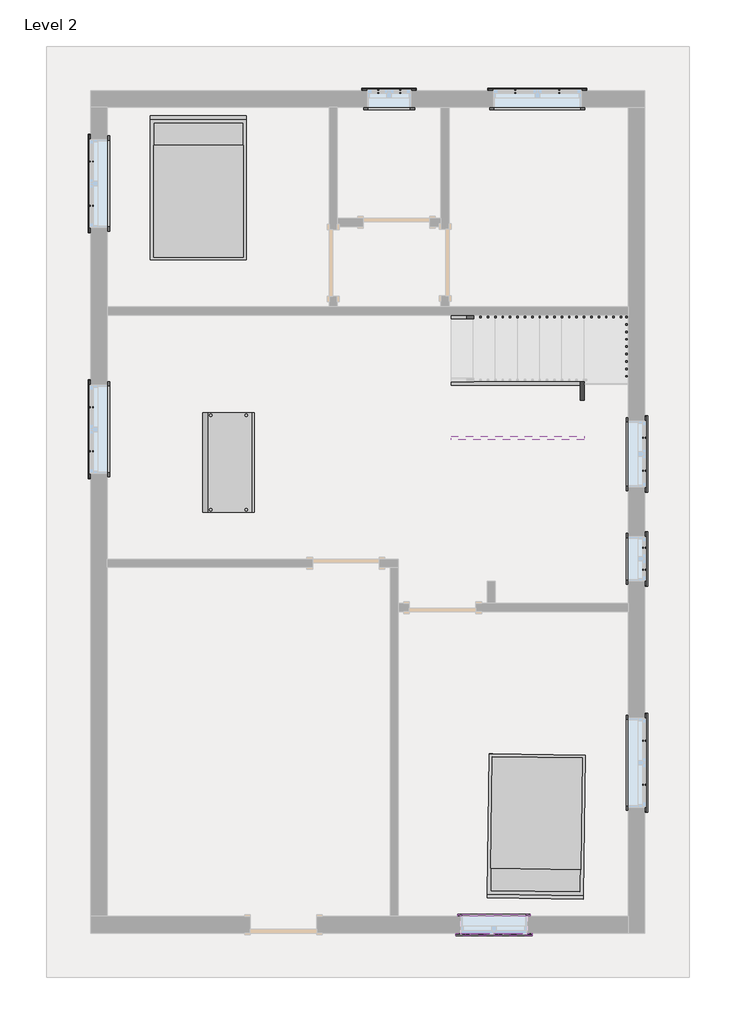
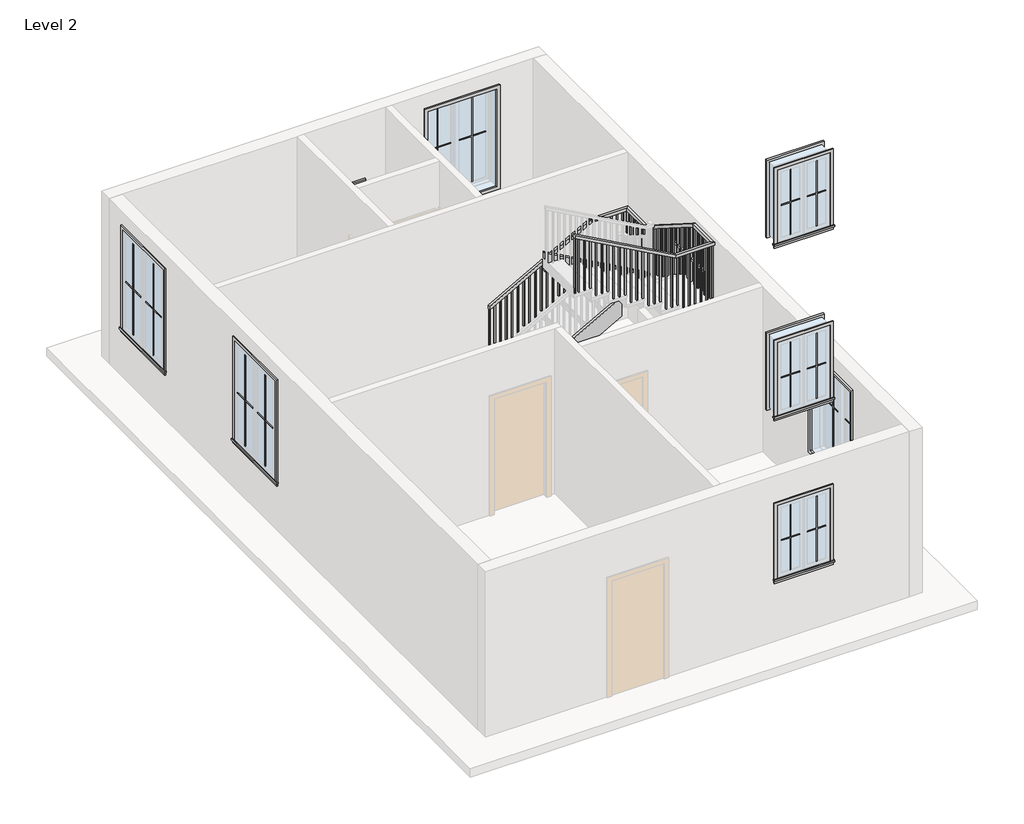
# One storey, part 2 of 2: 41 proxies, 3 members, 2 furniture elements, 1 railing.
"""IFC4 building model written with IfcOpenShell, lengths in millimetres."""

from ifc_helpers import new_model, si_unit, frame, origin, place, context, project, spatial, polyline, outline, extrude, faceted_brep, transform, mapped, element, save
from components import modern_coffee_table_17989_modern_coffee_table_17989_d3a860c8, muntin_pattern_2x2_muntin_pattern_2x2_2b4d9f72, muntin_pattern_2x2_muntin_pattern_2x2_ef995ed3, muntin_pattern_2x2_muntin_pattern_2x2_53152e2c, muntin_pattern_2x2_muntin_pattern_2x2_e8f3e573, muntin_pattern_2x2_muntin_pattern_2x2_9b64c8d5, muntin_pattern_2x2_muntin_pattern_2x2_d319fd2e, trim_window_exterior_flat_with_sill_b7e4d11c, trim_window_exterior_flat_with_sill_a665a915, trim_window_exterior_flat_with_sill_66148908, trim_window_interior_flat_picture_frame_936b8d2a, trim_window_interior_flat_picture_frame_d485c387, trim_window_interior_flat_picture_frame_d5b7f3a4, bed_17739_bed_17739_15c61121

model = new_model("IFC4")

# Units and contexts
model_context = context("Model", 3, world=origin())
ifc_project = project(units=[si_unit("LENGTHUNIT", "METRE", prefix="MILLI")], contexts=[model_context])

# Site, building, storey
site = spatial("IfcSite", under=ifc_project)
building = spatial("IfcBuilding", under=site)
storey = spatial("IfcBuildingStorey", under=building, Name="Level 2", Elevation=3048.0)

# Proxies
placement = place(None, origin())
modern_coffee_table_17989_modern_coffee_table_17989_shape = modern_coffee_table_17989_modern_coffee_table_17989_d3a860c8(model_context)
element("IfcBuildingElementProxy", 1, Name="Modern_Coffee_Table_17989 : Modern_Coffee_Table_17989", ObjectType="Modern_Coffee_Table_17989 : Modern_Coffee_Table_17989", at=placement, inside=storey, context=model_context, shape_type="MappedRepresentation", body=[
    mapped(modern_coffee_table_17989_modern_coffee_table_17989_shape, transform((3060.7, 9172.1823212, 3048.0), x_axis=(0.0, 1.0, 0.0), y_axis=(-1.0, 0.0, 0.0), z_axis=(0.0, 0.0, 1.0))),
])
muntin_pattern_2x2_muntin_pattern_2x2_shape = muntin_pattern_2x2_muntin_pattern_2x2_2b4d9f72(model_context)
element("IfcBuildingElementProxy", 2, Name="Muntin Pattern_2x2 : Muntin Pattern_2x2", ObjectType="Muntin Pattern_2x2 : Muntin Pattern_2x2", at=placement, inside=storey, context=model_context, shape_type="MappedRepresentation", body=[
    mapped(muntin_pattern_2x2_muntin_pattern_2x2_shape, transform((1533.525, 12477.4069306, 4032.25), x_axis=(0.0, 1.0, 0.0), y_axis=(-1.0, 0.0, 0.0), z_axis=(0.0, 0.0, 1.0))),
])
element("IfcBuildingElementProxy", 3, Name="Muntin Pattern_2x2 : Muntin Pattern_2x2", ObjectType="Muntin Pattern_2x2 : Muntin Pattern_2x2", at=placement, inside=storey, context=model_context, shape_type="MappedRepresentation", body=[
    mapped(muntin_pattern_2x2_muntin_pattern_2x2_shape, transform((7361.2375, 14045.8073212, 4032.25), x_axis=(1.0, 0.0, 0.0), y_axis=(0.0, 1.0, 0.0), z_axis=(0.0, 0.0, 1.0))),
])
element("IfcBuildingElementProxy", 4, Name="Muntin Pattern_2x2 : Muntin Pattern_2x2", ObjectType="Muntin Pattern_2x2 : Muntin Pattern_2x2", at=placement, inside=storey, context=model_context, shape_type="MappedRepresentation", body=[
    mapped(muntin_pattern_2x2_muntin_pattern_2x2_shape, transform((9134.475, 5119.2948212, 4032.25), x_axis=(0.0, -1.0, 0.0), y_axis=(1.0, 0.0, 0.0), z_axis=(0.0, 0.0, 1.0))),
])
element("IfcBuildingElementProxy", 5, Name="Muntin Pattern_2x2 : Muntin Pattern_2x2", ObjectType="Muntin Pattern_2x2 : Muntin Pattern_2x2", at=placement, inside=storey, context=model_context, shape_type="MappedRepresentation", body=[
    mapped(muntin_pattern_2x2_muntin_pattern_2x2_shape, transform((1533.525, 9097.5698212, 4032.25), x_axis=(0.0, 1.0, 0.0), y_axis=(-1.0, 0.0, 0.0), z_axis=(0.0, 0.0, 1.0))),
])
muntin_pattern_2x2_muntin_pattern_2x2_2_shape = muntin_pattern_2x2_muntin_pattern_2x2_ef995ed3(model_context)
element("IfcBuildingElementProxy", 6, Name="Muntin Pattern_2x2 : Muntin Pattern_2x2", ObjectType="Muntin Pattern_2x2 : Muntin Pattern_2x2", at=placement, inside=storey, context=model_context, shape_type="MappedRepresentation", body=[
    mapped(muntin_pattern_2x2_muntin_pattern_2x2_2_shape, transform((1533.525, 13083.8319306, 4032.25), x_axis=(0.0, -1.0, 0.0), y_axis=(1.0, 0.0, 0.0), z_axis=(0.0, 0.0, 1.0))),
])
element("IfcBuildingElementProxy", 7, Name="Muntin Pattern_2x2 : Muntin Pattern_2x2", ObjectType="Muntin Pattern_2x2 : Muntin Pattern_2x2", at=placement, inside=storey, context=model_context, shape_type="MappedRepresentation", body=[
    mapped(muntin_pattern_2x2_muntin_pattern_2x2_2_shape, transform((7967.6625, 14045.8073212, 4032.25), x_axis=(-1.0, 0.0, 0.0), y_axis=(0.0, -1.0, 0.0), z_axis=(0.0, 0.0, 1.0))),
])
element("IfcBuildingElementProxy", 8, Name="Muntin Pattern_2x2 : Muntin Pattern_2x2", ObjectType="Muntin Pattern_2x2 : Muntin Pattern_2x2", at=placement, inside=storey, context=model_context, shape_type="MappedRepresentation", body=[
    mapped(muntin_pattern_2x2_muntin_pattern_2x2_2_shape, transform((9134.475, 4512.8698212, 4032.25), x_axis=(0.0, 1.0, 0.0), y_axis=(-1.0, 0.0, 0.0), z_axis=(0.0, 0.0, 1.0))),
])
element("IfcBuildingElementProxy", 9, Name="Muntin Pattern_2x2 : Muntin Pattern_2x2", ObjectType="Muntin Pattern_2x2 : Muntin Pattern_2x2", at=placement, inside=storey, context=model_context, shape_type="MappedRepresentation", body=[
    mapped(muntin_pattern_2x2_muntin_pattern_2x2_2_shape, transform((1533.525, 9703.9948212, 4032.25), x_axis=(0.0, -1.0, 0.0), y_axis=(1.0, 0.0, 0.0), z_axis=(0.0, 0.0, 1.0))),
])
muntin_pattern_2x2_muntin_pattern_2x2_3_shape = muntin_pattern_2x2_muntin_pattern_2x2_53152e2c(model_context)
element("IfcBuildingElementProxy", 10, Name="Muntin Pattern_2x2 : Muntin Pattern_2x2", ObjectType="Muntin Pattern_2x2 : Muntin Pattern_2x2", at=placement, inside=storey, context=model_context, shape_type="MappedRepresentation", body=[
    mapped(muntin_pattern_2x2_muntin_pattern_2x2_3_shape, transform((9134.475, 7771.2135712, 4032.25), x_axis=(0.0, -1.0, 0.0), y_axis=(1.0, 0.0, 0.0), z_axis=(0.0, 0.0, 1.0))),
])
element("IfcBuildingElementProxy", 11, Name="Muntin Pattern_2x2 : Muntin Pattern_2x2", ObjectType="Muntin Pattern_2x2 : Muntin Pattern_2x2", at=placement, inside=storey, context=model_context, shape_type="MappedRepresentation", body=[
    mapped(muntin_pattern_2x2_muntin_pattern_2x2_3_shape, transform((5475.2875, 14045.8073212, 4032.25), x_axis=(1.0, 0.0, 0.0), y_axis=(0.0, 1.0, 0.0), z_axis=(0.0, 0.0, 1.0))),
])
muntin_pattern_2x2_muntin_pattern_2x2_4_shape = muntin_pattern_2x2_muntin_pattern_2x2_e8f3e573(model_context)
element("IfcBuildingElementProxy", 12, Name="Muntin Pattern_2x2 : Muntin Pattern_2x2", ObjectType="Muntin Pattern_2x2 : Muntin Pattern_2x2", at=placement, inside=storey, context=model_context, shape_type="MappedRepresentation", body=[
    mapped(muntin_pattern_2x2_muntin_pattern_2x2_4_shape, transform((9134.475, 7469.5885712, 4032.25), x_axis=(0.0, 1.0, 0.0), y_axis=(-1.0, 0.0, 0.0), z_axis=(0.0, 0.0, 1.0))),
])
element("IfcBuildingElementProxy", 13, Name="Muntin Pattern_2x2 : Muntin Pattern_2x2", ObjectType="Muntin Pattern_2x2 : Muntin Pattern_2x2", at=placement, inside=storey, context=model_context, shape_type="MappedRepresentation", body=[
    mapped(muntin_pattern_2x2_muntin_pattern_2x2_4_shape, transform((5776.9125, 14045.8073212, 4032.25), x_axis=(-1.0, 0.0, 0.0), y_axis=(0.0, -1.0, 0.0), z_axis=(0.0, 0.0, 1.0))),
])
muntin_pattern_2x2_muntin_pattern_2x2_5_shape = muntin_pattern_2x2_muntin_pattern_2x2_9b64c8d5(model_context)
element("IfcBuildingElementProxy", 14, Name="Muntin Pattern_2x2 : Muntin Pattern_2x2", ObjectType="Muntin Pattern_2x2 : Muntin Pattern_2x2", at=placement, inside=storey, context=model_context, shape_type="MappedRepresentation", body=[
    mapped(muntin_pattern_2x2_muntin_pattern_2x2_5_shape, transform((9134.475, 9287.1024384, 4032.25), x_axis=(0.0, -1.0, 0.0), y_axis=(1.0, 0.0, 0.0), z_axis=(0.0, 0.0, 1.0))),
])
element("IfcBuildingElementProxy", 15, Name="Muntin Pattern_2x2 : Muntin Pattern_2x2", ObjectType="Muntin Pattern_2x2 : Muntin Pattern_2x2", at=placement, inside=storey, context=model_context, shape_type="MappedRepresentation", body=[
    mapped(muntin_pattern_2x2_muntin_pattern_2x2_5_shape, transform((7294.5625, 2482.4573212, 4279.430542), x_axis=(-1.0, 0.0, 0.0), y_axis=(0.0, -1.0, 0.0), z_axis=(0.0, 0.0, 1.0))),
])
element("IfcBuildingElementProxy", 16, Name="Muntin Pattern_2x2 : Muntin Pattern_2x2", ObjectType="Muntin Pattern_2x2 : Muntin Pattern_2x2", at=placement, inside=storey, context=model_context, shape_type="MappedRepresentation", body=[
    mapped(muntin_pattern_2x2_muntin_pattern_2x2_5_shape, transform((7294.5625, 2482.4573212, 7281.2610953), x_axis=(-1.0, 0.0, 0.0), y_axis=(0.0, -1.0, 0.0), z_axis=(0.0, 0.0, 1.0))),
])
element("IfcBuildingElementProxy", 17, Name="Muntin Pattern_2x2 : Muntin Pattern_2x2", ObjectType="Muntin Pattern_2x2 : Muntin Pattern_2x2", at=placement, inside=storey, context=model_context, shape_type="MappedRepresentation", body=[
    mapped(muntin_pattern_2x2_muntin_pattern_2x2_5_shape, transform((7294.5625, 2482.4573212, 10461.9845423), x_axis=(-1.0, 0.0, 0.0), y_axis=(0.0, -1.0, 0.0), z_axis=(0.0, 0.0, 1.0))),
])
muntin_pattern_2x2_muntin_pattern_2x2_6_shape = muntin_pattern_2x2_muntin_pattern_2x2_d319fd2e(model_context)
element("IfcBuildingElementProxy", 18, Name="Muntin Pattern_2x2 : Muntin Pattern_2x2", ObjectType="Muntin Pattern_2x2 : Muntin Pattern_2x2", at=placement, inside=storey, context=model_context, shape_type="MappedRepresentation", body=[
    mapped(muntin_pattern_2x2_muntin_pattern_2x2_6_shape, transform((9134.475, 8833.0774384, 4032.25), x_axis=(0.0, 1.0, 0.0), y_axis=(-1.0, 0.0, 0.0), z_axis=(0.0, 0.0, 1.0))),
])
element("IfcBuildingElementProxy", 19, Name="Muntin Pattern_2x2 : Muntin Pattern_2x2", ObjectType="Muntin Pattern_2x2 : Muntin Pattern_2x2", at=placement, inside=storey, context=model_context, shape_type="MappedRepresentation", body=[
    mapped(muntin_pattern_2x2_muntin_pattern_2x2_6_shape, transform((6840.5375, 2482.4573212, 4279.430542), x_axis=(1.0, 0.0, 0.0), y_axis=(0.0, 1.0, 0.0), z_axis=(0.0, 0.0, 1.0))),
])
element("IfcBuildingElementProxy", 20, Name="Muntin Pattern_2x2 : Muntin Pattern_2x2", ObjectType="Muntin Pattern_2x2 : Muntin Pattern_2x2", at=placement, inside=storey, context=model_context, shape_type="MappedRepresentation", body=[
    mapped(muntin_pattern_2x2_muntin_pattern_2x2_6_shape, transform((6840.5375, 2482.4573212, 7281.2610953), x_axis=(1.0, 0.0, 0.0), y_axis=(0.0, 1.0, 0.0), z_axis=(0.0, 0.0, 1.0))),
])
element("IfcBuildingElementProxy", 21, Name="Muntin Pattern_2x2 : Muntin Pattern_2x2", ObjectType="Muntin Pattern_2x2 : Muntin Pattern_2x2", at=placement, inside=storey, context=model_context, shape_type="MappedRepresentation", body=[
    mapped(muntin_pattern_2x2_muntin_pattern_2x2_6_shape, transform((6840.5375, 2482.4573212, 10461.9845423), x_axis=(1.0, 0.0, 0.0), y_axis=(0.0, 1.0, 0.0), z_axis=(0.0, 0.0, 1.0))),
])
trim_window_exterior_flat_with_sill_shape = trim_window_exterior_flat_with_sill_b7e4d11c(model_context)
element("IfcBuildingElementProxy", 22, Name="Trim-Window-Exterior-Flat : with Sill", ObjectType="Trim-Window-Exterior-Flat : with Sill", at=placement, inside=storey, context=model_context, shape_type="MappedRepresentation", body=[
    mapped(trim_window_exterior_flat_with_sill_shape, transform((1524.0, 12780.6194306, 5791.2), x_axis=(0.0, -1.0, 0.0), y_axis=(0.0, 0.0, 1.0), z_axis=(-1.0, 0.0, 0.0))),
])
element("IfcBuildingElementProxy", 23, Name="Trim-Window-Exterior-Flat : with Sill", ObjectType="Trim-Window-Exterior-Flat : with Sill", at=placement, inside=storey, context=model_context, shape_type="MappedRepresentation", body=[
    mapped(trim_window_exterior_flat_with_sill_shape, transform((7664.45, 14055.3323212, 5791.2), x_axis=(-1.0, 0.0, 0.0), y_axis=(0.0, 0.0, 1.0), z_axis=(0.0, 1.0, 0.0))),
])
element("IfcBuildingElementProxy", 24, Name="Trim-Window-Exterior-Flat : with Sill", ObjectType="Trim-Window-Exterior-Flat : with Sill", at=placement, inside=storey, context=model_context, shape_type="MappedRepresentation", body=[
    mapped(trim_window_exterior_flat_with_sill_shape, transform((9144.0, 4816.0823212, 5791.2), x_axis=(0.0, 1.0, 0.0), y_axis=(0.0, 0.0, 1.0), z_axis=(1.0, 0.0, 0.0))),
])
element("IfcBuildingElementProxy", 25, Name="Trim-Window-Exterior-Flat : with Sill", ObjectType="Trim-Window-Exterior-Flat : with Sill", at=placement, inside=storey, context=model_context, shape_type="MappedRepresentation", body=[
    mapped(trim_window_exterior_flat_with_sill_shape, transform((1524.0, 9400.7823212, 5791.2), x_axis=(0.0, -1.0, 0.0), y_axis=(0.0, 0.0, 1.0), z_axis=(-1.0, 0.0, 0.0))),
])
trim_window_exterior_flat_with_sill_2_shape = trim_window_exterior_flat_with_sill_a665a915(model_context)
element("IfcBuildingElementProxy", 26, Name="Trim-Window-Exterior-Flat : with Sill", ObjectType="Trim-Window-Exterior-Flat : with Sill", at=placement, inside=storey, context=model_context, shape_type="MappedRepresentation", body=[
    mapped(trim_window_exterior_flat_with_sill_2_shape, transform((9144.0, 7620.4010712, 4876.8), x_axis=(0.0, 1.0, 0.0), y_axis=(0.0, 0.0, 1.0), z_axis=(1.0, 0.0, 0.0))),
])
element("IfcBuildingElementProxy", 27, Name="Trim-Window-Exterior-Flat : with Sill", ObjectType="Trim-Window-Exterior-Flat : with Sill", at=placement, inside=storey, context=model_context, shape_type="MappedRepresentation", body=[
    mapped(trim_window_exterior_flat_with_sill_2_shape, transform((5626.1, 14055.3323212, 4876.8), x_axis=(-1.0, 0.0, 0.0), y_axis=(0.0, 0.0, 1.0), z_axis=(0.0, 1.0, 0.0))),
])
trim_window_exterior_flat_with_sill_3_shape = trim_window_exterior_flat_with_sill_66148908(model_context)
element("IfcBuildingElementProxy", 28, Name="Trim-Window-Exterior-Flat : with Sill", ObjectType="Trim-Window-Exterior-Flat : with Sill", at=placement, inside=storey, context=model_context, shape_type="MappedRepresentation", body=[
    mapped(trim_window_exterior_flat_with_sill_3_shape, transform((9144.0, 9060.0899384, 5308.6), x_axis=(0.0, 1.0, 0.0), y_axis=(0.0, 0.0, 1.0), z_axis=(1.0, 0.0, 0.0))),
])
element("IfcBuildingElementProxy", 29, Name="Trim-Window-Exterior-Flat : with Sill", ObjectType="Trim-Window-Exterior-Flat : with Sill", at=placement, inside=storey, context=model_context, shape_type="MappedRepresentation", body=[
    mapped(trim_window_exterior_flat_with_sill_3_shape, transform((7067.55, 2472.9323212, 5555.780542), x_axis=(1.0, 0.0, 0.0), y_axis=(0.0, 0.0, 1.0), z_axis=(0.0, -1.0, 0.0))),
])
element("IfcBuildingElementProxy", 30, Name="Trim-Window-Exterior-Flat : with Sill", ObjectType="Trim-Window-Exterior-Flat : with Sill", at=placement, inside=storey, context=model_context, shape_type="MappedRepresentation", body=[
    mapped(trim_window_exterior_flat_with_sill_3_shape, transform((7067.55, 2472.9323212, 8557.6110953), x_axis=(1.0, 0.0, 0.0), y_axis=(0.0, 0.0, 1.0), z_axis=(0.0, -1.0, 0.0))),
])
element("IfcBuildingElementProxy", 31, Name="Trim-Window-Exterior-Flat : with Sill", ObjectType="Trim-Window-Exterior-Flat : with Sill", at=placement, inside=storey, context=model_context, shape_type="MappedRepresentation", body=[
    mapped(trim_window_exterior_flat_with_sill_3_shape, transform((7067.55, 2472.9323212, 11738.3345423), x_axis=(1.0, 0.0, 0.0), y_axis=(0.0, 0.0, 1.0), z_axis=(0.0, -1.0, 0.0))),
])
trim_window_interior_flat_picture_frame_shape = trim_window_interior_flat_picture_frame_936b8d2a(model_context)
element("IfcBuildingElementProxy", 32, Name="Trim-Window-Interior-Flat : Picture Frame", ObjectType="Trim-Window-Interior-Flat : Picture Frame", at=placement, inside=storey, context=model_context, shape_type="MappedRepresentation", body=[
    mapped(trim_window_interior_flat_picture_frame_shape, transform((1752.6, 12780.6194306, 5791.2), x_axis=(0.0, 1.0, 0.0), y_axis=(0.0, 0.0, 1.0), z_axis=(1.0, 0.0, 0.0))),
])
element("IfcBuildingElementProxy", 33, Name="Trim-Window-Interior-Flat : Picture Frame", ObjectType="Trim-Window-Interior-Flat : Picture Frame", at=placement, inside=storey, context=model_context, shape_type="MappedRepresentation", body=[
    mapped(trim_window_interior_flat_picture_frame_shape, transform((7664.45, 13826.7323212, 5791.2), x_axis=(1.0, 0.0, 0.0), y_axis=(0.0, 0.0, 1.0), z_axis=(0.0, -1.0, 0.0))),
])
element("IfcBuildingElementProxy", 34, Name="Trim-Window-Interior-Flat : Picture Frame", ObjectType="Trim-Window-Interior-Flat : Picture Frame", at=placement, inside=storey, context=model_context, shape_type="MappedRepresentation", body=[
    mapped(trim_window_interior_flat_picture_frame_shape, transform((8915.4, 4816.0823212, 5791.2), x_axis=(0.0, -1.0, 0.0), y_axis=(0.0, 0.0, 1.0), z_axis=(-1.0, 0.0, 0.0))),
])
element("IfcBuildingElementProxy", 35, Name="Trim-Window-Interior-Flat : Picture Frame", ObjectType="Trim-Window-Interior-Flat : Picture Frame", at=placement, inside=storey, context=model_context, shape_type="MappedRepresentation", body=[
    mapped(trim_window_interior_flat_picture_frame_shape, transform((1752.6, 9400.7823212, 5791.2), x_axis=(0.0, 1.0, 0.0), y_axis=(0.0, 0.0, 1.0), z_axis=(1.0, 0.0, 0.0))),
])
trim_window_interior_flat_picture_frame_2_shape = trim_window_interior_flat_picture_frame_d485c387(model_context)
element("IfcBuildingElementProxy", 36, Name="Trim-Window-Interior-Flat : Picture Frame", ObjectType="Trim-Window-Interior-Flat : Picture Frame", at=placement, inside=storey, context=model_context, shape_type="MappedRepresentation", body=[
    mapped(trim_window_interior_flat_picture_frame_2_shape, transform((8915.4, 7620.4010712, 4876.8), x_axis=(0.0, -1.0, 0.0), y_axis=(0.0, 0.0, 1.0), z_axis=(-1.0, 0.0, 0.0))),
])
element("IfcBuildingElementProxy", 37, Name="Trim-Window-Interior-Flat : Picture Frame", ObjectType="Trim-Window-Interior-Flat : Picture Frame", at=placement, inside=storey, context=model_context, shape_type="MappedRepresentation", body=[
    mapped(trim_window_interior_flat_picture_frame_2_shape, transform((5626.1, 13826.7323212, 4876.8), x_axis=(1.0, 0.0, 0.0), y_axis=(0.0, 0.0, 1.0), z_axis=(0.0, -1.0, 0.0))),
])
trim_window_interior_flat_picture_frame_3_shape = trim_window_interior_flat_picture_frame_d5b7f3a4(model_context)
element("IfcBuildingElementProxy", 38, Name="Trim-Window-Interior-Flat : Picture Frame", ObjectType="Trim-Window-Interior-Flat : Picture Frame", at=placement, inside=storey, context=model_context, shape_type="MappedRepresentation", body=[
    mapped(trim_window_interior_flat_picture_frame_3_shape, transform((8915.4, 9060.0899384, 5308.6), x_axis=(0.0, -1.0, 0.0), y_axis=(0.0, 0.0, 1.0), z_axis=(-1.0, 0.0, 0.0))),
])
element("IfcBuildingElementProxy", 39, Name="Trim-Window-Interior-Flat : Picture Frame", ObjectType="Trim-Window-Interior-Flat : Picture Frame", at=placement, inside=storey, context=model_context, shape_type="MappedRepresentation", body=[
    mapped(trim_window_interior_flat_picture_frame_3_shape, transform((7067.55, 2701.5323212, 5555.780542), x_axis=(-1.0, 0.0, 0.0), y_axis=(0.0, 0.0, 1.0), z_axis=(0.0, 1.0, 0.0))),
])
element("IfcBuildingElementProxy", 40, Name="Trim-Window-Interior-Flat : Picture Frame", ObjectType="Trim-Window-Interior-Flat : Picture Frame", at=placement, inside=storey, context=model_context, shape_type="MappedRepresentation", body=[
    mapped(trim_window_interior_flat_picture_frame_3_shape, transform((7067.55, 2701.5323212, 8557.6110953), x_axis=(-1.0, 0.0, 0.0), y_axis=(0.0, 0.0, 1.0), z_axis=(0.0, 1.0, 0.0))),
])
element("IfcBuildingElementProxy", 41, Name="Trim-Window-Interior-Flat : Picture Frame", ObjectType="Trim-Window-Interior-Flat : Picture Frame", at=placement, inside=storey, context=model_context, shape_type="MappedRepresentation", body=[
    mapped(trim_window_interior_flat_picture_frame_3_shape, transform((7067.55, 2701.5323212, 11738.3345423), x_axis=(-1.0, 0.0, 0.0), y_axis=(0.0, 0.0, 1.0), z_axis=(0.0, 1.0, 0.0))),
])

# Furniture
bed_17739_bed_17739_shape = bed_17739_bed_17739_15c61121(model_context)
element("IfcFurniture", 42, ObjectType="Bed_17739 : Bed_17739", at=placement, inside=storey, context=model_context, shape_type="MappedRepresentation", body=[
    mapped(bed_17739_bed_17739_shape, transform((3003.55, 12696.4323212, 3048.0), x_axis=(1.0, 0.0, 0.0), y_axis=(0.0, 1.0, 0.0), z_axis=(0.0, 0.0, 1.0))),
])
element("IfcFurniture", 43, ObjectType="Bed_17739 : Bed_17739", at=placement, inside=storey, context=model_context, shape_type="MappedRepresentation", body=[
    mapped(bed_17739_bed_17739_shape, transform((7650.1504891, 3963.5673274, 3048.0), x_axis=(-0.9999063358908578, 0.013686469424921632, 0.0), y_axis=(-0.013686469424921632, -0.9999063358908578, 0.0), z_axis=(0.0, 0.0, 1.0))),
])

# Members
element("IfcMember", 44, ObjectType="Stringer - 2\" Width", at=placement, inside=storey, context=model_context, shape_type="SweptSolid", body=[
    extrude(outline(polyline([(3255.5983948, 6477.0), (3048.0, 6477.0), (3048.0, 6730.9445028), (3894.6974984, 8255.0), (4243.3761726, 8255.0), (3255.5983948, 6477.0)])), frame((0.0, 10004.0323212, 0.0), z_axis=(0.0, 1.0, 0.0), x_axis=(0.0, 0.0, 1.0)), (0.0, 0.0, 1.0), 50.8),
])
element("IfcMember", 45, ObjectType="Stringer - 2\" Width", at=placement, inside=storey, context=model_context, shape_type="SweptSolid", body=[
    extrude(outline(polyline([(10054.8323212, 4448.2030053), (10054.8323212, 4087.1566026), (9305.5323212, 4562.9026344), (9305.5323212, 4923.949037), (10054.8323212, 4448.2030053)])), frame((8255.0, 0.0, 0.0), z_axis=(1.0, 0.0, 0.0), x_axis=(0.0, 1.0, 0.0)), (0.0, 0.0, 1.0), 50.8),
])
element("IfcMember", 46, ObjectType="Stringer - 2\" Width", at=placement, inside=storey, context=model_context, shape_type="SweptSolid", body=[
    extrude(outline(polyline([(4769.5863873, 8305.8), (5118.2650614, 8305.8), (6134.2650614, 6477.0), (5785.5863873, 6477.0), (4769.5863873, 8305.8)])), frame((0.0, 9254.7323212, 0.0), z_axis=(0.0, 1.0, 0.0), x_axis=(0.0, 0.0, 1.0)), (0.0, 0.0, 1.0), 50.8),
])

# Railing
element("IfcRailing", 47, ObjectType="Handrail - Rectangular", at=placement, inside=storey, context=model_context, shape_type="SolidModel", body=[
    faceted_brep([(6477.0, 10969.2323212, 4131.7333333), (6477.0, 10969.2323212, 4073.620221), (6477.0, 10918.4323212, 4073.620221), (6477.0, 10918.4323212, 4131.7333333), (8242.3, 10969.2323212, 5112.4555556), (8255.4636022, 10969.2323212, 5061.6555556), (8255.4636022, 10918.4323212, 5061.6555556), (8242.3, 10918.4323212, 5112.4555556), (8915.4, 10969.2323212, 5112.4555556), (8915.4, 10969.2323212, 5061.6555556), (8864.6, 10918.4323212, 5061.6555556), (8864.6, 10918.4323212, 5112.4555556), (8915.4, 10377.0948212, 5112.4555556), (8915.4, 10362.3301405, 5061.6555556), (8864.6, 10362.3301405, 5061.6555556), (8864.6, 10377.0948212, 5112.4555556), (8915.4, 8932.4698212, 6029.6777778), (8915.4, 8917.7051405, 5978.8777778), (8864.6, 8917.7051405, 5978.8777778), (8864.6, 8932.4698212, 6029.6777778), (8915.4, 8340.3323212, 6029.6777778), (8915.4, 8340.3323212, 5978.8777778), (8864.6, 8391.1323212, 5978.8777778), (8864.6, 8391.1323212, 6029.6777778), (8242.3, 8340.3323212, 6029.6777778), (8229.1363978, 8340.3323212, 5978.8777778), (8229.1363978, 8391.1323212, 5978.8777778), (8242.3, 8391.1323212, 6029.6777778), (6477.0, 8340.3323212, 7010.4), (6477.0, 8391.1323212, 7010.4), (6477.0, 8391.1323212, 6952.2868876), (6477.0, 8340.3323212, 6952.2868876)], [[[0, 1, 2, 3]], [[1, 0, 4, 5]], [[2, 1, 5, 6]], [[3, 2, 6, 7]], [[0, 3, 7, 4]], [[5, 4, 8, 9]], [[6, 5, 9, 10]], [[7, 6, 10, 11]], [[4, 7, 11, 8]], [[9, 8, 12, 13]], [[10, 9, 13, 14]], [[11, 10, 14, 15]], [[8, 11, 15, 12]], [[13, 12, 16, 17]], [[14, 13, 17, 18]], [[15, 14, 18, 19]], [[12, 15, 19, 16]], [[17, 16, 20, 21]], [[18, 17, 21, 22]], [[19, 18, 22, 23]], [[16, 19, 23, 20]], [[21, 20, 24, 25]], [[22, 21, 25, 26]], [[23, 22, 26, 27]], [[20, 23, 27, 24]], [[28, 29, 30, 31]], [[25, 24, 28, 31]], [[26, 25, 31, 30]], [[27, 26, 30, 29]], [[24, 27, 29, 28]]]),
    extrude(outline(polyline([(6915.245221, 6543.675), (5926.6666667, 6543.675), (5926.6666667, 6562.725), (6904.6618876, 6562.725), (6915.245221, 6543.675)])), frame((0.0, 8356.2073212, 0.0), z_axis=(0.0, 1.0, 0.0), x_axis=(0.0, 0.0, 1.0)), (0.0, 0.0, 1.0), 19.05),
    extrude(outline(polyline([(6858.8007765, 6645.275), (5926.6666667, 6645.275), (5926.6666667, 6664.325), (6848.2174432, 6664.325), (6858.8007765, 6645.275)])), frame((0.0, 8356.2073212, 0.0), z_axis=(0.0, 1.0, 0.0), x_axis=(0.0, 0.0, 1.0)), (0.0, 0.0, 1.0), 19.05),
    extrude(outline(polyline([(6802.3563321, 6746.875), (5926.6666667, 6746.875), (5926.6666667, 6765.925), (6791.7729988, 6765.925), (6802.3563321, 6746.875)])), frame((0.0, 8356.2073212, 0.0), z_axis=(0.0, 1.0, 0.0), x_axis=(0.0, 0.0, 1.0)), (0.0, 0.0, 1.0), 19.05),
    extrude(outline(polyline([(6745.9118876, 6848.475), (5757.3333333, 6848.475), (5757.3333333, 6867.525), (6735.3285543, 6867.525), (6745.9118876, 6848.475)])), frame((0.0, 8356.2073212, 0.0), z_axis=(0.0, 1.0, 0.0), x_axis=(0.0, 0.0, 1.0)), (0.0, 0.0, 1.0), 19.05),
    extrude(outline(polyline([(6689.4674432, 6950.075), (5757.3333333, 6950.075), (5757.3333333, 6969.125), (6678.8841099, 6969.125), (6689.4674432, 6950.075)])), frame((0.0, 8356.2073212, 0.0), z_axis=(0.0, 1.0, 0.0), x_axis=(0.0, 0.0, 1.0)), (0.0, 0.0, 1.0), 19.05),
    extrude(outline(polyline([(6633.0229988, 7051.675), (5757.3333333, 7051.675), (5757.3333333, 7070.725), (6622.4396654, 7070.725), (6633.0229988, 7051.675)])), frame((0.0, 8356.2073212, 0.0), z_axis=(0.0, 1.0, 0.0), x_axis=(0.0, 0.0, 1.0)), (0.0, 0.0, 1.0), 19.05),
    extrude(outline(polyline([(6576.5785543, 7153.275), (5588.0, 7153.275), (5588.0, 7172.325), (6565.995221, 7172.325), (6576.5785543, 7153.275)])), frame((0.0, 8356.2073212, 0.0), z_axis=(0.0, 1.0, 0.0), x_axis=(0.0, 0.0, 1.0)), (0.0, 0.0, 1.0), 19.05),
    extrude(outline(polyline([(6520.1341099, 7254.875), (5588.0, 7254.875), (5588.0, 7273.925), (6509.5507765, 7273.925), (6520.1341099, 7254.875)])), frame((0.0, 8356.2073212, 0.0), z_axis=(0.0, 1.0, 0.0), x_axis=(0.0, 0.0, 1.0)), (0.0, 0.0, 1.0), 19.05),
    extrude(outline(polyline([(6463.6896654, 7356.475), (5588.0, 7356.475), (5588.0, 7375.525), (6453.1063321, 7375.525), (6463.6896654, 7356.475)])), frame((0.0, 8356.2073212, 0.0), z_axis=(0.0, 1.0, 0.0), x_axis=(0.0, 0.0, 1.0)), (0.0, 0.0, 1.0), 19.05),
    extrude(outline(polyline([(6407.245221, 7458.075), (5418.6666667, 7458.075), (5418.6666667, 7477.125), (6396.6618876, 7477.125), (6407.245221, 7458.075)])), frame((0.0, 8356.2073212, 0.0), z_axis=(0.0, 1.0, 0.0), x_axis=(0.0, 0.0, 1.0)), (0.0, 0.0, 1.0), 19.05),
    extrude(outline(polyline([(6350.8007765, 7559.675), (5418.6666667, 7559.675), (5418.6666667, 7578.725), (6340.2174432, 7578.725), (6350.8007765, 7559.675)])), frame((0.0, 8356.2073212, 0.0), z_axis=(0.0, 1.0, 0.0), x_axis=(0.0, 0.0, 1.0)), (0.0, 0.0, 1.0), 19.05),
    extrude(outline(polyline([(6294.3563321, 7661.275), (5418.6666667, 7661.275), (5418.6666667, 7680.325), (6283.7729988, 7680.325), (6294.3563321, 7661.275)])), frame((0.0, 8356.2073212, 0.0), z_axis=(0.0, 1.0, 0.0), x_axis=(0.0, 0.0, 1.0)), (0.0, 0.0, 1.0), 19.05),
    extrude(outline(polyline([(6237.9118876, 7762.875), (5249.3333333, 7762.875), (5249.3333333, 7781.925), (6227.3285543, 7781.925), (6237.9118876, 7762.875)])), frame((0.0, 8356.2073212, 0.0), z_axis=(0.0, 1.0, 0.0), x_axis=(0.0, 0.0, 1.0)), (0.0, 0.0, 1.0), 19.05),
    extrude(outline(polyline([(6181.4674432, 7864.475), (5249.3333333, 7864.475), (5249.3333333, 7883.525), (6170.8841099, 7883.525), (6181.4674432, 7864.475)])), frame((0.0, 8356.2073212, 0.0), z_axis=(0.0, 1.0, 0.0), x_axis=(0.0, 0.0, 1.0)), (0.0, 0.0, 1.0), 19.05),
    extrude(outline(polyline([(6125.0229988, 7966.075), (5249.3333333, 7966.075), (5249.3333333, 7985.125), (6114.4396654, 7985.125), (6125.0229988, 7966.075)])), frame((0.0, 8356.2073212, 0.0), z_axis=(0.0, 1.0, 0.0), x_axis=(0.0, 0.0, 1.0)), (0.0, 0.0, 1.0), 19.05),
    extrude(outline(polyline([(6068.5785543, 8067.675), (5080.0, 8067.675), (5080.0, 8086.725), (6057.995221, 8086.725), (6068.5785543, 8067.675)])), frame((0.0, 8356.2073212, 0.0), z_axis=(0.0, 1.0, 0.0), x_axis=(0.0, 0.0, 1.0)), (0.0, 0.0, 1.0), 19.05),
    extrude(outline(polyline([(6012.1341099, 8169.275), (5080.0, 8169.275), (5080.0, 8188.325), (6001.5507765, 8188.325), (6012.1341099, 8169.275)])), frame((0.0, 8356.2073212, 0.0), z_axis=(0.0, 1.0, 0.0), x_axis=(0.0, 0.0, 1.0)), (0.0, 0.0, 1.0), 19.05),
    extrude(outline(polyline([(8289.925, 8356.2073212), (8270.875, 8356.2073212), (8270.875, 8375.2573212), (8289.925, 8375.2573212), (8289.925, 8356.2073212)])), frame((0.0, 0.0, 5080.0), z_axis=(0.0, 0.0, 1.0), x_axis=(1.0, 0.0, 0.0)), (0.0, 0.0, 1.0), 898.8777778),
    extrude(outline(polyline([(8391.525, 8356.2073212), (8372.475, 8356.2073212), (8372.475, 8375.2573212), (8391.525, 8375.2573212), (8391.525, 8356.2073212)])), frame((0.0, 0.0, 4910.6666667), z_axis=(0.0, 0.0, 1.0), x_axis=(1.0, 0.0, 0.0)), (0.0, 0.0, 1.0), 1068.2111111),
    extrude(outline(polyline([(8493.125, 8356.2073212), (8474.075, 8356.2073212), (8474.075, 8375.2573212), (8493.125, 8375.2573212), (8493.125, 8356.2073212)])), frame((0.0, 0.0, 4910.6666667), z_axis=(0.0, 0.0, 1.0), x_axis=(1.0, 0.0, 0.0)), (0.0, 0.0, 1.0), 1068.2111111),
    extrude(outline(polyline([(8594.725, 8356.2073212), (8575.675, 8356.2073212), (8575.675, 8375.2573212), (8594.725, 8375.2573212), (8594.725, 8356.2073212)])), frame((0.0, 0.0, 4910.6666667), z_axis=(0.0, 0.0, 1.0), x_axis=(1.0, 0.0, 0.0)), (0.0, 0.0, 1.0), 1068.2111111),
    extrude(outline(polyline([(8696.325, 8356.2073212), (8677.275, 8356.2073212), (8677.275, 8375.2573212), (8696.325, 8375.2573212), (8696.325, 8356.2073212)])), frame((0.0, 0.0, 4910.6666667), z_axis=(0.0, 0.0, 1.0), x_axis=(1.0, 0.0, 0.0)), (0.0, 0.0, 1.0), 1068.2111111),
    extrude(outline(polyline([(8797.925, 8356.2073212), (8778.875, 8356.2073212), (8778.875, 8375.2573212), (8797.925, 8375.2573212), (8797.925, 8356.2073212)])), frame((0.0, 0.0, 4910.6666667), z_axis=(0.0, 0.0, 1.0), x_axis=(1.0, 0.0, 0.0)), (0.0, 0.0, 1.0), 1068.2111111),
    extrude(outline(polyline([(8899.525, 8413.3573212), (8899.525, 8394.3073212), (8880.475, 8394.3073212), (8880.475, 8413.3573212), (8899.525, 8413.3573212)])), frame((0.0, 0.0, 4910.6666667), z_axis=(0.0, 0.0, 1.0), x_axis=(1.0, 0.0, 0.0)), (0.0, 0.0, 1.0), 1068.2111111),
    extrude(outline(polyline([(8899.525, 8514.9573212), (8899.525, 8495.9073212), (8880.475, 8495.9073212), (8880.475, 8514.9573212), (8899.525, 8514.9573212)])), frame((0.0, 0.0, 4910.6666667), z_axis=(0.0, 0.0, 1.0), x_axis=(1.0, 0.0, 0.0)), (0.0, 0.0, 1.0), 1068.2111111),
    extrude(outline(polyline([(8899.525, 8616.5573212), (8899.525, 8597.5073212), (8880.475, 8597.5073212), (8880.475, 8616.5573212), (8899.525, 8616.5573212)])), frame((0.0, 0.0, 4910.6666667), z_axis=(0.0, 0.0, 1.0), x_axis=(1.0, 0.0, 0.0)), (0.0, 0.0, 1.0), 1068.2111111),
    extrude(outline(polyline([(8899.525, 8718.1573212), (8899.525, 8699.1073212), (8880.475, 8699.1073212), (8880.475, 8718.1573212), (8899.525, 8718.1573212)])), frame((0.0, 0.0, 4910.6666667), z_axis=(0.0, 0.0, 1.0), x_axis=(1.0, 0.0, 0.0)), (0.0, 0.0, 1.0), 1068.2111111),
    extrude(outline(polyline([(8899.525, 8819.7573212), (8899.525, 8800.7073212), (8880.475, 8800.7073212), (8880.475, 8819.7573212), (8899.525, 8819.7573212)])), frame((0.0, 0.0, 4910.6666667), z_axis=(0.0, 0.0, 1.0), x_axis=(1.0, 0.0, 0.0)), (0.0, 0.0, 1.0), 1068.2111111),
    extrude(outline(polyline([(8899.525, 8921.3573212), (8899.525, 8902.3073212), (8880.475, 8902.3073212), (8880.475, 8921.3573212), (8899.525, 8921.3573212)])), frame((0.0, 0.0, 4910.6666667), z_axis=(0.0, 0.0, 1.0), x_axis=(1.0, 0.0, 0.0)), (0.0, 0.0, 1.0), 1068.2111111),
    extrude(outline(polyline([(9022.9573212, 5912.0509964), (9022.9573212, 4910.6666667), (9003.9073212, 4910.6666667), (9003.9073212, 5924.1462345), (9022.9573212, 5912.0509964)])), frame((8880.475, 0.0, 0.0), z_axis=(1.0, 0.0, 0.0), x_axis=(0.0, 1.0, 0.0)), (0.0, 0.0, 1.0), 19.05),
    extrude(outline(polyline([(9124.5573212, 5847.5430599), (9124.5573212, 4910.6666667), (9105.5073212, 4910.6666667), (9105.5073212, 5859.638298), (9124.5573212, 5847.5430599)])), frame((8880.475, 0.0, 0.0), z_axis=(1.0, 0.0, 0.0), x_axis=(0.0, 1.0, 0.0)), (0.0, 0.0, 1.0), 19.05),
    extrude(outline(polyline([(9226.1573212, 5783.0351234), (9226.1573212, 4910.6666667), (9207.1073212, 4910.6666667), (9207.1073212, 5795.1303615), (9226.1573212, 5783.0351234)])), frame((8880.475, 0.0, 0.0), z_axis=(1.0, 0.0, 0.0), x_axis=(0.0, 1.0, 0.0)), (0.0, 0.0, 1.0), 19.05),
    extrude(outline(polyline([(9327.7573212, 5718.5271869), (9327.7573212, 4741.3333333), (9308.7073212, 4741.3333333), (9308.7073212, 5730.622425), (9327.7573212, 5718.5271869)])), frame((8880.475, 0.0, 0.0), z_axis=(1.0, 0.0, 0.0), x_axis=(0.0, 1.0, 0.0)), (0.0, 0.0, 1.0), 19.05),
    extrude(outline(polyline([(9429.3573212, 5654.0192504), (9429.3573212, 4741.3333333), (9410.3073212, 4741.3333333), (9410.3073212, 5666.1144884), (9429.3573212, 5654.0192504)])), frame((8880.475, 0.0, 0.0), z_axis=(1.0, 0.0, 0.0), x_axis=(0.0, 1.0, 0.0)), (0.0, 0.0, 1.0), 19.05),
    extrude(outline(polyline([(9530.9573212, 5589.5113138), (9530.9573212, 4572.0), (9511.9073212, 4572.0), (9511.9073212, 5601.6065519), (9530.9573212, 5589.5113138)])), frame((8880.475, 0.0, 0.0), z_axis=(1.0, 0.0, 0.0), x_axis=(0.0, 1.0, 0.0)), (0.0, 0.0, 1.0), 19.05),
    extrude(outline(polyline([(9632.5573212, 5525.0033773), (9632.5573212, 4572.0), (9613.5073212, 4572.0), (9613.5073212, 5537.0986154), (9632.5573212, 5525.0033773)])), frame((8880.475, 0.0, 0.0), z_axis=(1.0, 0.0, 0.0), x_axis=(0.0, 1.0, 0.0)), (0.0, 0.0, 1.0), 19.05),
    extrude(outline(polyline([(9734.1573212, 5460.4954408), (9734.1573212, 4572.0), (9715.1073212, 4572.0), (9715.1073212, 5472.5906789), (9734.1573212, 5460.4954408)])), frame((8880.475, 0.0, 0.0), z_axis=(1.0, 0.0, 0.0), x_axis=(0.0, 1.0, 0.0)), (0.0, 0.0, 1.0), 19.05),
    extrude(outline(polyline([(9835.7573212, 5395.9875043), (9835.7573212, 4402.6666667), (9816.7073212, 4402.6666667), (9816.7073212, 5408.0827424), (9835.7573212, 5395.9875043)])), frame((8880.475, 0.0, 0.0), z_axis=(1.0, 0.0, 0.0), x_axis=(0.0, 1.0, 0.0)), (0.0, 0.0, 1.0), 19.05),
    extrude(outline(polyline([(9937.3573212, 5331.4795678), (9937.3573212, 4402.6666667), (9918.3073212, 4402.6666667), (9918.3073212, 5343.5748059), (9937.3573212, 5331.4795678)])), frame((8880.475, 0.0, 0.0), z_axis=(1.0, 0.0, 0.0), x_axis=(0.0, 1.0, 0.0)), (0.0, 0.0, 1.0), 19.05),
    extrude(outline(polyline([(10038.9573212, 5266.9716313), (10038.9573212, 4402.6666667), (10019.9073212, 4402.6666667), (10019.9073212, 5279.0668694), (10038.9573212, 5266.9716313)])), frame((8880.475, 0.0, 0.0), z_axis=(1.0, 0.0, 0.0), x_axis=(0.0, 1.0, 0.0)), (0.0, 0.0, 1.0), 19.05),
    extrude(outline(polyline([(10140.5573212, 5202.4636948), (10140.5573212, 4233.3333333), (10121.5073212, 4233.3333333), (10121.5073212, 5214.5589329), (10140.5573212, 5202.4636948)])), frame((8880.475, 0.0, 0.0), z_axis=(1.0, 0.0, 0.0), x_axis=(0.0, 1.0, 0.0)), (0.0, 0.0, 1.0), 19.05),
    extrude(outline(polyline([(10242.1573212, 5137.9557583), (10242.1573212, 4233.3333333), (10223.1073212, 4233.3333333), (10223.1073212, 5150.0509964), (10242.1573212, 5137.9557583)])), frame((8880.475, 0.0, 0.0), z_axis=(1.0, 0.0, 0.0), x_axis=(0.0, 1.0, 0.0)), (0.0, 0.0, 1.0), 19.05),
    extrude(outline(polyline([(10343.7573212, 5073.4478218), (10343.7573212, 4233.3333333), (10324.7073212, 4233.3333333), (10324.7073212, 5085.5430599), (10343.7573212, 5073.4478218)])), frame((8880.475, 0.0, 0.0), z_axis=(1.0, 0.0, 0.0), x_axis=(0.0, 1.0, 0.0)), (0.0, 0.0, 1.0), 19.05),
    extrude(outline(polyline([(8899.525, 10445.3573212), (8899.525, 10426.3073212), (8880.475, 10426.3073212), (8880.475, 10445.3573212), (8899.525, 10445.3573212)])), frame((0.0, 0.0, 4233.3333333), z_axis=(0.0, 0.0, 1.0), x_axis=(1.0, 0.0, 0.0)), (0.0, 0.0, 1.0), 828.3222222),
    extrude(outline(polyline([(8899.525, 10546.9573212), (8899.525, 10527.9073212), (8880.475, 10527.9073212), (8880.475, 10546.9573212), (8899.525, 10546.9573212)])), frame((0.0, 0.0, 4233.3333333), z_axis=(0.0, 0.0, 1.0), x_axis=(1.0, 0.0, 0.0)), (0.0, 0.0, 1.0), 828.3222222),
    extrude(outline(polyline([(8899.525, 10648.5573212), (8899.525, 10629.5073212), (8880.475, 10629.5073212), (8880.475, 10648.5573212), (8899.525, 10648.5573212)])), frame((0.0, 0.0, 4233.3333333), z_axis=(0.0, 0.0, 1.0), x_axis=(1.0, 0.0, 0.0)), (0.0, 0.0, 1.0), 828.3222222),
    extrude(outline(polyline([(8899.525, 10750.1573212), (8899.525, 10731.1073212), (8880.475, 10731.1073212), (8880.475, 10750.1573212), (8899.525, 10750.1573212)])), frame((0.0, 0.0, 4233.3333333), z_axis=(0.0, 0.0, 1.0), x_axis=(1.0, 0.0, 0.0)), (0.0, 0.0, 1.0), 828.3222222),
    extrude(outline(polyline([(8899.525, 10851.7573212), (8899.525, 10832.7073212), (8880.475, 10832.7073212), (8880.475, 10851.7573212), (8899.525, 10851.7573212)])), frame((0.0, 0.0, 4233.3333333), z_axis=(0.0, 0.0, 1.0), x_axis=(1.0, 0.0, 0.0)), (0.0, 0.0, 1.0), 828.3222222),
    extrude(outline(polyline([(8804.275, 10953.3573212), (8823.325, 10953.3573212), (8823.325, 10934.3073212), (8804.275, 10934.3073212), (8804.275, 10953.3573212)])), frame((0.0, 0.0, 4233.3333333), z_axis=(0.0, 0.0, 1.0), x_axis=(1.0, 0.0, 0.0)), (0.0, 0.0, 1.0), 828.3222222),
    extrude(outline(polyline([(8702.675, 10953.3573212), (8721.725, 10953.3573212), (8721.725, 10934.3073212), (8702.675, 10934.3073212), (8702.675, 10953.3573212)])), frame((0.0, 0.0, 4233.3333333), z_axis=(0.0, 0.0, 1.0), x_axis=(1.0, 0.0, 0.0)), (0.0, 0.0, 1.0), 828.3222222),
    extrude(outline(polyline([(8601.075, 10953.3573212), (8620.125, 10953.3573212), (8620.125, 10934.3073212), (8601.075, 10934.3073212), (8601.075, 10953.3573212)])), frame((0.0, 0.0, 4233.3333333), z_axis=(0.0, 0.0, 1.0), x_axis=(1.0, 0.0, 0.0)), (0.0, 0.0, 1.0), 828.3222222),
    extrude(outline(polyline([(8499.475, 10953.3573212), (8518.525, 10953.3573212), (8518.525, 10934.3073212), (8499.475, 10934.3073212), (8499.475, 10953.3573212)])), frame((0.0, 0.0, 4233.3333333), z_axis=(0.0, 0.0, 1.0), x_axis=(1.0, 0.0, 0.0)), (0.0, 0.0, 1.0), 828.3222222),
    extrude(outline(polyline([(8397.875, 10953.3573212), (8416.925, 10953.3573212), (8416.925, 10934.3073212), (8397.875, 10934.3073212), (8397.875, 10953.3573212)])), frame((0.0, 0.0, 4233.3333333), z_axis=(0.0, 0.0, 1.0), x_axis=(1.0, 0.0, 0.0)), (0.0, 0.0, 1.0), 828.3222222),
    extrude(outline(polyline([(8296.275, 10953.3573212), (8315.325, 10953.3573212), (8315.325, 10934.3073212), (8296.275, 10934.3073212), (8296.275, 10953.3573212)])), frame((0.0, 0.0, 4233.3333333), z_axis=(0.0, 0.0, 1.0), x_axis=(1.0, 0.0, 0.0)), (0.0, 0.0, 1.0), 828.3222222),
    extrude(outline(polyline([(5027.8841099, 8194.675), (4064.0, 8194.675), (4064.0, 8213.725), (5038.4674432, 8213.725), (5027.8841099, 8194.675)])), frame((0.0, 10934.3073212, 0.0), z_axis=(0.0, 1.0, 0.0), x_axis=(0.0, 0.0, 1.0)), (0.0, 0.0, 1.0), 19.05),
    extrude(outline(polyline([(4971.4396654, 8093.075), (4064.0, 8093.075), (4064.0, 8112.125), (4982.0229988, 8112.125), (4971.4396654, 8093.075)])), frame((0.0, 10934.3073212, 0.0), z_axis=(0.0, 1.0, 0.0), x_axis=(0.0, 0.0, 1.0)), (0.0, 0.0, 1.0), 19.05),
    extrude(outline(polyline([(4914.995221, 7991.475), (4064.0, 7991.475), (4064.0, 8010.525), (4925.5785543, 8010.525), (4914.995221, 7991.475)])), frame((0.0, 10934.3073212, 0.0), z_axis=(0.0, 1.0, 0.0), x_axis=(0.0, 0.0, 1.0)), (0.0, 0.0, 1.0), 19.05),
    extrude(outline(polyline([(4858.5507765, 7889.875), (3894.6666667, 7889.875), (3894.6666667, 7908.925), (4869.1341099, 7908.925), (4858.5507765, 7889.875)])), frame((0.0, 10934.3073212, 0.0), z_axis=(0.0, 1.0, 0.0), x_axis=(0.0, 0.0, 1.0)), (0.0, 0.0, 1.0), 19.05),
    extrude(outline(polyline([(4802.1063321, 7788.275), (3894.6666667, 7788.275), (3894.6666667, 7807.325), (4812.6896654, 7807.325), (4802.1063321, 7788.275)])), frame((0.0, 10934.3073212, 0.0), z_axis=(0.0, 1.0, 0.0), x_axis=(0.0, 0.0, 1.0)), (0.0, 0.0, 1.0), 19.05),
    extrude(outline(polyline([(4745.6618876, 7686.675), (3894.6666667, 7686.675), (3894.6666667, 7705.725), (4756.245221, 7705.725), (4745.6618876, 7686.675)])), frame((0.0, 10934.3073212, 0.0), z_axis=(0.0, 1.0, 0.0), x_axis=(0.0, 0.0, 1.0)), (0.0, 0.0, 1.0), 19.05),
    extrude(outline(polyline([(4689.2174432, 7585.075), (3725.3333333, 7585.075), (3725.3333333, 7604.125), (4699.8007765, 7604.125), (4689.2174432, 7585.075)])), frame((0.0, 10934.3073212, 0.0), z_axis=(0.0, 1.0, 0.0), x_axis=(0.0, 0.0, 1.0)), (0.0, 0.0, 1.0), 19.05),
    extrude(outline(polyline([(4632.7729988, 7483.475), (3725.3333333, 7483.475), (3725.3333333, 7502.525), (4643.3563321, 7502.525), (4632.7729988, 7483.475)])), frame((0.0, 10934.3073212, 0.0), z_axis=(0.0, 1.0, 0.0), x_axis=(0.0, 0.0, 1.0)), (0.0, 0.0, 1.0), 19.05),
    extrude(outline(polyline([(4576.3285543, 7381.875), (3725.3333333, 7381.875), (3725.3333333, 7400.925), (4586.9118876, 7400.925), (4576.3285543, 7381.875)])), frame((0.0, 10934.3073212, 0.0), z_axis=(0.0, 1.0, 0.0), x_axis=(0.0, 0.0, 1.0)), (0.0, 0.0, 1.0), 19.05),
    extrude(outline(polyline([(4519.8841099, 7280.275), (3556.0, 7280.275), (3556.0, 7299.325), (4530.4674432, 7299.325), (4519.8841099, 7280.275)])), frame((0.0, 10934.3073212, 0.0), z_axis=(0.0, 1.0, 0.0), x_axis=(0.0, 0.0, 1.0)), (0.0, 0.0, 1.0), 19.05),
    extrude(outline(polyline([(4463.4396654, 7178.675), (3556.0, 7178.675), (3556.0, 7197.725), (4474.0229988, 7197.725), (4463.4396654, 7178.675)])), frame((0.0, 10934.3073212, 0.0), z_axis=(0.0, 1.0, 0.0), x_axis=(0.0, 0.0, 1.0)), (0.0, 0.0, 1.0), 19.05),
    extrude(outline(polyline([(4406.995221, 7077.075), (3556.0, 7077.075), (3556.0, 7096.125), (4417.5785543, 7096.125), (4406.995221, 7077.075)])), frame((0.0, 10934.3073212, 0.0), z_axis=(0.0, 1.0, 0.0), x_axis=(0.0, 0.0, 1.0)), (0.0, 0.0, 1.0), 19.05),
    extrude(outline(polyline([(4350.5507765, 6975.475), (3386.6666667, 6975.475), (3386.6666667, 6994.525), (4361.1341099, 6994.525), (4350.5507765, 6975.475)])), frame((0.0, 10934.3073212, 0.0), z_axis=(0.0, 1.0, 0.0), x_axis=(0.0, 0.0, 1.0)), (0.0, 0.0, 1.0), 19.05),
    extrude(outline(polyline([(4294.1063321, 6873.875), (3386.6666667, 6873.875), (3386.6666667, 6892.925), (4304.6896654, 6892.925), (4294.1063321, 6873.875)])), frame((0.0, 10934.3073212, 0.0), z_axis=(0.0, 1.0, 0.0), x_axis=(0.0, 0.0, 1.0)), (0.0, 0.0, 1.0), 19.05),
    extrude(outline(polyline([(4237.6618876, 6772.275), (3386.6666667, 6772.275), (3386.6666667, 6791.325), (4248.245221, 6791.325), (4237.6618876, 6772.275)])), frame((0.0, 10934.3073212, 0.0), z_axis=(0.0, 1.0, 0.0), x_axis=(0.0, 0.0, 1.0)), (0.0, 0.0, 1.0), 19.05),
    extrude(outline(polyline([(4181.2174432, 6670.675), (3217.3333333, 6670.675), (3217.3333333, 6689.725), (4191.8007765, 6689.725), (4181.2174432, 6670.675)])), frame((0.0, 10934.3073212, 0.0), z_axis=(0.0, 1.0, 0.0), x_axis=(0.0, 0.0, 1.0)), (0.0, 0.0, 1.0), 19.05),
    extrude(outline(polyline([(4124.7729988, 6569.075), (3217.3333333, 6569.075), (3217.3333333, 6588.125), (4135.3563321, 6588.125), (4124.7729988, 6569.075)])), frame((0.0, 10934.3073212, 0.0), z_axis=(0.0, 1.0, 0.0), x_axis=(0.0, 0.0, 1.0)), (0.0, 0.0, 1.0), 19.05),
    extrude(outline(polyline([(8899.525, 8375.2573212), (8899.525, 8356.2073212), (8880.475, 8356.2073212), (8880.475, 8375.2573212), (8899.525, 8375.2573212)])), frame((0.0, 0.0, 4910.6666667), z_axis=(0.0, 0.0, 1.0), x_axis=(1.0, 0.0, 0.0)), (0.0, 0.0, 1.0), 1068.2111111),
    extrude(outline(polyline([(8880.475, 10953.3573212), (8899.525, 10953.3573212), (8899.525, 10934.3073212), (8880.475, 10934.3073212), (8880.475, 10953.3573212)])), frame((0.0, 0.0, 4233.3333333), z_axis=(0.0, 0.0, 1.0), x_axis=(1.0, 0.0, 0.0)), (0.0, 0.0, 1.0), 828.3222222),
    extrude(outline(polyline([(6952.2868876, 6477.0), (5926.6666667, 6477.0), (5926.6666667, 6496.05), (6941.7035543, 6496.05), (6952.2868876, 6477.0)])), frame((0.0, 8356.2073212, 0.0), z_axis=(0.0, 1.0, 0.0), x_axis=(0.0, 0.0, 1.0)), (0.0, 0.0, 1.0), 19.05),
    extrude(outline(polyline([(4073.620221, 6477.0), (3217.3333333, 6477.0), (3217.3333333, 6496.05), (4084.2035543, 6496.05), (4073.620221, 6477.0)])), frame((0.0, 10934.3073212, 0.0), z_axis=(0.0, 1.0, 0.0), x_axis=(0.0, 0.0, 1.0)), (0.0, 0.0, 1.0), 19.05),
])

save(model, "model.ifc")

# Revit data of these elements
# Type "Modern_Coffee_Table_17989 : Modern_Coffee_Table_17989"
#   Default Elevation = 0
# Type "Muntin Pattern_2x2 : Muntin Pattern_2x2"
#   Width [instance default] = 4' - 0"
#   Thickness = 0' - 0 1/2"
#   Height [instance default] = 4' - 0"
#   Distance = 0' - 0 3/4"
#   Interior Material [instance default] = none
#   Exterior Material [instance default] = none
#   Default Elevation = 0
# Type "Trim-Window-Exterior-Flat : with Sill"
#   Trim Width = 0' - 2 1/4"
#   Trim Thickness_Picture Frame = 0' - 1 1/4"
#   Trim Thickness_with Sill = 0' - 0 3/4"
#   Sill Thickness = 0' - 1 1/4"
#   Opening Width [instance default] = 2' - 0"
#   Opening Height [instance default] = 3' - 0"
#   Default Elevation = 4' - 0"
#   Sill = yes
#   Picture Frame = no
#   Trim Material [instance default] = none
# Type "Trim-Window-Interior-Flat : Picture Frame"
#   Trim Thickness_Picture Frame = 0' - 1 1/4"
#   Trim Width = 0' - 2 1/4"
#   Trim Thickness_with Sill = 0' - 0 3/4"
#   Sill Thickness = 0' - 1 1/4"
#   Opening Width [instance default] = 2' - 0"
#   Opening Height [instance default] = 3' - 0"
#   Default Elevation = 4' - 0"
#   Sill = no
#   Picture Frame = yes
#   Trim Material [instance default] = none
# Type "Bed_17739 : Bed_17739"
#   Default Elevation = 0
# Type "Handrail - Rectangular"
#   Assembly Code = "C2010400"
#   built-in parameter 1008612 = 0.0416667 (stored number, unit not read)
#   built-in parameter 1008611 = 0.0416667 (stored number, unit not read)
#   built-in parameter 1008609 = 0.333333 (stored number, unit not read)
#   built-in parameter 1008604 = 0.166667 (stored number, unit not read)
#   built-in parameter 1008603 = 0.166667 (stored number, unit not read)
#   Railing Height = 3' - 0"
#   built-in parameter 1008630 = 2
#   built-in parameter 1008610 = 2
#   built-in parameter 1008618 = Baluster - Square : 3/4"
# Element 1 (IfcBuildingElementProxy, "Modern_Coffee_Table_17989 : Modern_Coffee_Table_17989")
#   Phase Created = New Construction
#   Materials on its faces: "1 Wood", "1 Glass", "1 Metal"
# Elements 2, 3, 4, 5, 6, 7, 8, 9 (IfcBuildingElementProxy, "Muntin Pattern_2x2 : Muntin Pattern_2x2")
#   Width = 1' - 6 5/8"
#   Height = 5' - 6 1/2"
#   Interior Material = Wood - Stained
#   Exterior Material = Clad - White
#   Phase Created = New Construction
#   Materials on its faces: "Clad - White", "Wood - Stained"
# Elements 10, 11, 12, 13 (IfcBuildingElementProxy, "Muntin Pattern_2x2 : Muntin Pattern_2x2")
#   Width = 0' - 6 5/8"
#   Height = 2' - 6 1/2"
#   Interior Material = Wood - Stained
#   Exterior Material = Clad - White
#   Phase Created = New Construction
#   Materials on its faces: "Clad - White", "Wood - Stained"
# Elements 14, 15, 16, 17, 18, 19, 20, 21 (IfcBuildingElementProxy, "Muntin Pattern_2x2 : Muntin Pattern_2x2")
#   Width = 1' - 0 5/8"
#   Height = 3' - 11 1/2"
#   Interior Material = Wood - Stained
#   Exterior Material = Clad - White
#   Phase Created = New Construction
#   Materials on its faces: "Clad - White", "Wood - Stained"
# Elements 22, 23, 24, 25 (IfcBuildingElementProxy, "Trim-Window-Exterior-Flat : with Sill")
#   Opening Width = 4' - 0"
#   Opening Height = 6' - 0"
#   Trim Material = Clad - White
#   Phase Created = New Construction
#   Materials on its faces: "Clad - White"
# Elements 26, 27 (IfcBuildingElementProxy, "Trim-Window-Exterior-Flat : with Sill")
#   Opening Width = 2' - 0"
#   Opening Height = 3' - 0"
#   Trim Material = Clad - White
#   Phase Created = New Construction
#   Materials on its faces: "Clad - White"
# Elements 28, 29, 30, 31 (IfcBuildingElementProxy, "Trim-Window-Exterior-Flat : with Sill")
#   Opening Width = 3' - 0"
#   Opening Height = 4' - 5"
#   Trim Material = Clad - White
#   Phase Created = New Construction
#   Materials on its faces: "Clad - White"
# Elements 32, 33, 34, 35 (IfcBuildingElementProxy, "Trim-Window-Interior-Flat : Picture Frame")
#   Opening Width = 4' - 0"
#   Opening Height = 6' - 0"
#   Trim Material = Wood - Stained
#   Phase Created = New Construction
#   Materials on its faces: "Wood - Stained"
# Elements 36, 37 (IfcBuildingElementProxy, "Trim-Window-Interior-Flat : Picture Frame")
#   Opening Width = 2' - 0"
#   Opening Height = 3' - 0"
#   Trim Material = Wood - Stained
#   Phase Created = New Construction
#   Materials on its faces: "Wood - Stained"
# Elements 38, 39, 40, 41 (IfcBuildingElementProxy, "Trim-Window-Interior-Flat : Picture Frame")
#   Opening Width = 3' - 0"
#   Opening Height = 4' - 5"
#   Trim Material = Wood - Stained
#   Phase Created = New Construction
#   Materials on its faces: "Wood - Stained"
# Elements 42, 43 (IfcFurniture, "Bed_17739 : Bed_17739")
#   Phase Created = New Construction
#   Materials on its faces: "legs", "sheets", "bed frame", "Blanket"
# Elements 44, 45, 46 (IfcMember, "Stringer - 2\" Width")
#   Phase Created = New Construction
# Element 47 (IfcRailing, "Handrail - Rectangular")
#   Phase Created = New Construction
# Materials
#   "1 Wood": class "Glass", colour RGB 81 52 39, transparency 0, Cost = 0
#   "1 Glass": class "Glass", colour RGB 236 240 239, transparency 0.85, Cost = 0
#   "1 Metal": class "Glass", colour RGB 244 244 244, transparency 0, Cost = 0
#   "Clad - White": class "Wood", colour RGB 242 242 238, transparency 0, Cost = 0
#   "Wood - Stained": class "Wood", colour RGB 224 178 126, transparency 0, Cost = 0
#   "legs": colour RGB 90 73 37, transparency 0, Cost = 0
#   "sheets": colour RGB 200 195 176, transparency 0, Cost = 0
#   "bed frame": colour RGB 90 73 37, transparency 0, Cost = 0
#   "Blanket": class "System", colour RGB 59 0 1, transparency 0, Cost = 0
